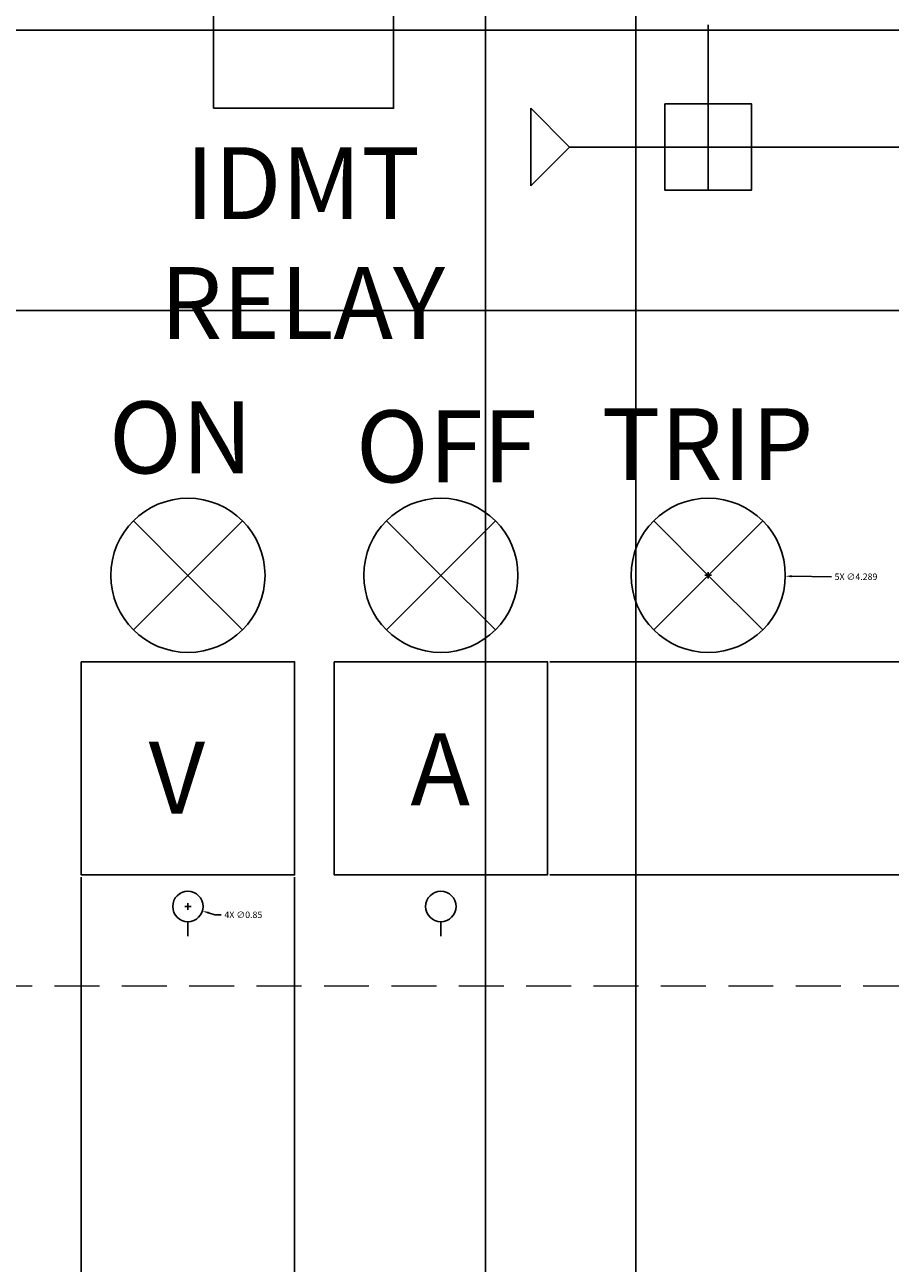
# Model space of a CAD drawing. Units: inches. Extents: x 412 to 584, y 208 to 437.
# Tile 19 of 28: x 471 to 495, y 352 to 387. Entities that reach past the tile are written whole.
import ezdxf

# ---------------------------------------------------------------- set-up
doc = ezdxf.new("R2010")
doc.units = ezdxf.units.IN
doc.header["$MEASUREMENT"] = 0
doc.linetypes.add('HIDDEN', pattern=[0.375, 0.25, -0.125])
for name, color, linetype, lineweight in [('A-ANNO-DIMS', 2, 'Continuous', 18), ('E-ANNO-TEXT', 7, 'Continuous', 18), ('E-ENCL-HIDN', 3, 'HIDDEN', 18), ('E-POWR-EQPM', 3, 'Continuous', 25)]:
    doc.layers.add(name, color=color, linetype=linetype, lineweight=lineweight)
doc.styles.get("Standard").update_dxf_attribs({"font": 'arial.ttf'})
doc.dimstyles.get("Standard").update_dxf_attribs({"dimtxt": 0.18, "dimasz": 0.18, "dimexe": 0.18, "dimexo": 0.0625, "dimgap": 0.09, "dimtad": 0, "dimtih": 1, "dimtoh": 1, "dimdec": 4, "dimzin": 0, "dimdsep": 46, "dimtxsty": 'Standard', "dimcen": 0.09, "dimadec": 0, "dimazin": 0, "dimtfac": 1, "dimtdec": 4, "dimtofl": 0, "dimtmove": 0, "dimatfit": 3, "dimfxl": 1, "dimtolj": 1, "dimtzin": 0, "dimarcsym": 0})

# ---------------------------------------------------------------- blocks, each defined once
blk = doc.blocks.new('*U1')
blk.add_line((0.758, -0.758), (-0.758, 0.758))
blk = doc.blocks.new('*U2')
at = {"color": 0, "linetype": 'ByBlock', "lineweight": -2, "transparency": 16777216}
blk.add_blockref('*U1', (78.828, 13.791), dxfattribs=at)
for p, rotation in [((80.344, 13.791), 269.9999999999999), ((78.828, 12.275), 89.99999999999996), ((80.344, 12.275), 180)]:
    blk.add_blockref('*U1', p, dxfattribs=dict(at, rotation=rotation))
blk = doc.blocks.new('INDICATOR-LAMP')
blk.add_circle((2.145, 2.145), 2.145)
at = {"rotation": 90.00000000000003}
blk.add_blockref('*U2', (15.178, -77.441), dxfattribs=at)
blk = doc.blocks.new('METER-VA')
blk.add_line((2.966, 0.398), (2.966, 0))
blk.add_lwpolyline([(0, 7.63), (5.932, 7.63), (5.932, 1.698), (0, 1.698)], close=True)
blk.add_circle((2.966, 0.821), 0.423)
blk = doc.blocks.new('*D23')
at = {"layer": 'A-ANNO-DIMS', "color": 0, "lineweight": -2, "transparency": 16777216}
for p, q in [((466.041, 360.196), (412.276, 360.196)), ((412.456, 360.016), (412.456, 354.967)), ((412.456, 349.553), (412.456, 354.603)), ((499.225, 349.373), (412.276, 349.373))]:
    blk.add_line(p, q, dxfattribs=at)
at = {"layer": 'A-ANNO-DIMS', "color": 0, "transparency": 16777216}
for points in [[(412.426, 360.016), (412.486, 360.016), (412.456, 360.196)], [(412.426, 349.553), (412.486, 349.553), (412.456, 349.373)]]:
    blk.add_solid(points, dxfattribs=at)
at = {"layer": 'Defpoints', "color": 0, "transparency": 16777216}
for p in [(466.104, 360.196), (412.456, 349.373), (499.288, 349.373)]:
    blk.add_point(p, dxfattribs=at)
at = {"layer": 'A-ANNO-DIMS', "color": 0, "transparency": 16777216, "insert": (412.456, 354.785), "char_height": 0.18, "attachment_point": 5}
blk.add_mtext('\\A1;10.823', dxfattribs=at)
blk = doc.blocks.new('*D28')
at = {"layer": 'A-ANNO-DIMS', "color": 0, "lineweight": -2, "transparency": 16777216}
for p, q in [((450.562, 256.635), (450.562, 437.465)), ((450.742, 437.285), (502.724, 437.285)), ((555.616, 437.285), (503.634, 437.285)), ((555.796, 256.635), (555.796, 437.465))]:
    blk.add_line(p, q, dxfattribs=at)
at = {"layer": 'A-ANNO-DIMS', "color": 0, "transparency": 16777216}
for points in [[(450.742, 437.315), (450.742, 437.255), (450.562, 437.285)], [(555.616, 437.315), (555.616, 437.255), (555.796, 437.285)]]:
    blk.add_solid(points, dxfattribs=at)
at = {"layer": 'Defpoints', "color": 0, "transparency": 16777216}
for p in [(555.796, 437.285), (450.562, 256.573), (555.796, 256.573)]:
    blk.add_point(p, dxfattribs=at)
at = {"layer": 'A-ANNO-DIMS', "color": 0, "transparency": 16777216, "insert": (503.179, 437.285), "char_height": 0.18, "attachment_point": 5}
blk.add_mtext('\\A1;105.23', dxfattribs=at)
blk = doc.blocks.new('*D30')
at = {"layer": 'A-ANNO-DIMS', "color": 0, "lineweight": -2, "transparency": 16777216}
for p, q in [((495.864, 386.793), (412.276, 386.793)), ((412.456, 386.613), (412.456, 383.072)), ((412.456, 379.167), (412.456, 382.708)), ((495.864, 378.987), (412.276, 378.987))]:
    blk.add_line(p, q, dxfattribs=at)
at = {"layer": 'A-ANNO-DIMS', "color": 0, "transparency": 16777216}
for points in [[(412.426, 386.613), (412.486, 386.613), (412.456, 386.793)], [(412.426, 379.167), (412.486, 379.167), (412.456, 378.987)]]:
    blk.add_solid(points, dxfattribs=at)
at = {"layer": 'Defpoints', "color": 0, "transparency": 16777216}
for p in [(495.927, 386.793), (412.456, 378.987), (495.927, 378.987)]:
    blk.add_point(p, dxfattribs=at)
at = {"layer": 'A-ANNO-DIMS', "color": 0, "transparency": 16777216, "insert": (412.456, 382.89), "char_height": 0.18, "attachment_point": 5}
blk.add_mtext('\\A1;7.807', dxfattribs=at)
blk = doc.blocks.new('*D33')
at = {"layer": 'A-ANNO-DIMS', "color": 0, "lineweight": -2, "transparency": 16777216}
for p, q in [((472.49, 363.226), (472.49, 208.233)), ((478.422, 363.226), (478.422, 208.233)), ((472.67, 208.413), (475.064, 208.413)), ((478.242, 208.413), (475.849, 208.413))]:
    blk.add_line(p, q, dxfattribs=at)
at = {"layer": 'A-ANNO-DIMS', "color": 0, "transparency": 16777216}
for points in [[(472.67, 208.443), (472.67, 208.383), (472.49, 208.413)], [(478.242, 208.443), (478.242, 208.383), (478.422, 208.413)]]:
    blk.add_solid(points, dxfattribs=at)
at = {"layer": 'Defpoints', "color": 0, "transparency": 16777216}
for p in [(472.49, 363.289), (478.422, 363.289), (478.422, 208.413)]:
    blk.add_point(p, dxfattribs=at)
at = {"layer": 'A-ANNO-DIMS', "color": 0, "transparency": 16777216, "insert": (475.456, 208.413), "char_height": 0.18, "attachment_point": 5}
blk.add_mtext('\\A1;5.932', dxfattribs=at)
blk = doc.blocks.new('*D35')
at = {"layer": 'A-ANNO-DIMS', "color": 0, "lineweight": -2, "transparency": 16777216}
for p, q in [((485.523, 369.221), (583.674, 369.221)), ((583.494, 369.041), (583.494, 366.437)), ((583.494, 363.469), (583.494, 366.073)), ((485.523, 363.289), (583.674, 363.289))]:
    blk.add_line(p, q, dxfattribs=at)
at = {"layer": 'A-ANNO-DIMS', "color": 0, "transparency": 16777216}
for points in [[(583.464, 369.041), (583.524, 369.041), (583.494, 369.221)], [(583.464, 363.469), (583.524, 363.469), (583.494, 363.289)]]:
    blk.add_solid(points, dxfattribs=at)
at = {"layer": 'Defpoints', "color": 0, "transparency": 16777216}
for p in [(485.46, 369.221), (485.46, 363.289), (583.494, 363.289)]:
    blk.add_point(p, dxfattribs=at)
at = {"layer": 'A-ANNO-DIMS', "color": 0, "transparency": 16777216, "insert": (583.494, 366.255), "char_height": 0.18, "attachment_point": 5}
blk.add_mtext('\\A1;5.932', dxfattribs=at)
blk = doc.blocks.new('*D41')
at = {"layer": 'A-ANNO-DIMS', "color": 0, "lineweight": -2, "transparency": 16777216}
for p, q in [((483.735, 316.045), (483.735, 437.465)), ((483.915, 437.285), (485.429, 437.285)), ((487.737, 437.285), (486.222, 437.285)), ((487.917, 316.045), (487.917, 437.465))]:
    blk.add_line(p, q, dxfattribs=at)
at = {"layer": 'A-ANNO-DIMS', "color": 0, "transparency": 16777216}
for points in [[(483.915, 437.315), (483.915, 437.255), (483.735, 437.285)], [(487.737, 437.315), (487.737, 437.255), (487.917, 437.285)]]:
    blk.add_solid(points, dxfattribs=at)
at = {"layer": 'Defpoints', "color": 0, "transparency": 16777216}
for p in [(487.917, 437.285), (483.735, 315.982), (487.917, 315.982)]:
    blk.add_point(p, dxfattribs=at)
at = {"layer": 'A-ANNO-DIMS', "color": 0, "transparency": 16777216, "insert": (485.826, 437.285), "char_height": 0.18, "attachment_point": 5}
blk.add_mtext('\\A1;4.182', dxfattribs=at)
blk = doc.blocks.new('*D43')
at = {"layer": 'A-ANNO-DIMS', "color": 0, "lineweight": -2, "transparency": 16777216}
for p, q in [((489.842, 371.624), (490.022, 371.624)), ((489.932, 371.534), (489.932, 371.714)), ((493.363, 371.585), (492.256, 371.598))]:
    blk.add_line(p, q, dxfattribs=at)
at = {"layer": 'A-ANNO-DIMS', "color": 0, "transparency": 16777216}
blk.add_solid([(492.257, 371.628), (492.256, 371.568), (492.076, 371.6)], dxfattribs=at)
at = {"layer": 'Defpoints', "color": 0, "transparency": 16777216}
for p in [(487.788, 371.648), (492.076, 371.6)]:
    blk.add_point(p, dxfattribs=at)
at = {"layer": 'A-ANNO-DIMS', "color": 0, "transparency": 16777216, "insert": (494.044, 371.585), "char_height": 0.18, "attachment_point": 5}
blk.add_mtext('\\A1;5X ∅4.289', dxfattribs=at)
blk = doc.blocks.new('*D49')
at = {"layer": 'A-ANNO-DIMS', "color": 0, "lineweight": -2, "transparency": 16777216}
for p, q in [((475.456, 362.322), (475.456, 362.502)), ((475.366, 362.412), (475.546, 362.412)), ((476.205, 362.181), (476.033, 362.234)), ((476.385, 362.181), (476.205, 362.181))]:
    blk.add_line(p, q, dxfattribs=at)
at = {"layer": 'A-ANNO-DIMS', "color": 0, "transparency": 16777216}
blk.add_solid([(476.041, 362.263), (476.024, 362.206), (475.861, 362.287)], dxfattribs=at)
at = {"layer": 'Defpoints', "color": 0, "transparency": 16777216}
for p in [(475.052, 362.538), (475.861, 362.287)]:
    blk.add_point(p, dxfattribs=at)
at = {"layer": 'A-ANNO-DIMS', "color": 0, "transparency": 16777216, "insert": (476.999, 362.181), "char_height": 0.18, "attachment_point": 5}
blk.add_mtext('\\A1;4X ∅0.85', dxfattribs=at)

msp = doc.modelspace()

# ---------------------------------------------------------------- linework, layer by layer
at = {"layer": 'E-ENCL-HIDN', "ltscale": 5}
msp.add_lwpolyline([(466.1037, 400.175), (538.6186, 400.175), (538.6186, 360.1961), (466.1037, 360.1961)], close=True, dxfattribs=at)
at = {"layer": 'E-POWR-EQPM'}
for p, q in [((489.932, 382.3348), (489.932, 386.939)), ((486.0745, 383.5382), (484.9955, 384.6173)), ((484.9955, 382.4592), (484.9955, 384.6173)), ((486.0745, 383.5382), (484.9955, 382.4592)), ((490.5891, 383.5382), (486.0745, 383.5382)), ((498.5775, 383.5382), (490.5891, 383.5382))]:
    msp.add_line(p, q, dxfattribs=at)
for points in [[(476.1684, 384.6173), (481.1791, 384.6173), (481.1791, 388.3577), (476.1684, 388.3577)], [(488.7286, 384.7417), (491.1355, 384.7417), (491.1355, 382.3348), (488.7286, 382.3348)]]:
    msp.add_lwpolyline(points, close=True, dxfattribs=at)

# ---------------------------------------------------------------- block references
at = {"layer": 'E-POWR-EQPM', "rotation": 270}
for p in [(473.3118, 373.7686), (480.3498, 373.7686), (487.7874, 373.7686)]:
    msp.add_blockref('INDICATOR-LAMP', p, dxfattribs=at)
at = {"layer": 'E-POWR-EQPM'}
for p in [(472.49, 361.591), (479.528, 361.591)]:
    msp.add_blockref('METER-VA', p, dxfattribs=at)

# ---------------------------------------------------------------- texts
at = {"layer": 'E-ANNO-TEXT', "char_height": 2, "attachment_point": 1}
for s, width, heights, insert in [('\\pxqc;IDMT\\PRELAY', 14.172159, [6.5789], (471.5606, 383.533)), ('\\pxqc;ON', 13.633448, [2.9648], (468.4413, 376.4612)), ('\\pxqc;OFF', 13.633448, [2.9648], (475.8321, 376.2109)), ('\\pxqc;TRIP', 13.633448, [2.9648], (483.0976, 376.2735)), ('\\pxqc;V', 13.633448, [2.9648], (468.3315, 366.9952)), ('\\pxqc;A', 13.633448, [2.9648], (475.659, 367.2276))]:
    msp.add_mtext_dynamic_manual_height_columns(s, width=width, gutter_width=1, heights=heights, dxfattribs=dict(at, insert=insert))

# ---------------------------------------------------------------- dimensions: what is measured, and where the dimension line sits
at = {"layer": 'A-ANNO-DIMS'}
for base, p1, p2, override, picture, middle in [((555.7959, 437.2847), (450.562, 256.5729), (555.7959, 256.5729), {"dimdec": 2, "dimlfac": 1, "dimrnd": 0, "dimzin": 0, "dimdsep": 46, "dimlunit": 2}, '*D28', (503.1789, 437.2847)), ((487.9167, 437.2847), (483.7347, 315.9821), (487.9167, 315.9821), {"dimdec": 3, "dimlfac": 1, "dimrnd": 0, "dimzin": 0, "dimdsep": 46, "dimlunit": 2}, '*D41', (485.8257, 437.2847)), ((478.4225, 208.4133), (472.4903, 363.2888), (478.4225, 363.2888), {"dimdec": 3, "dimlfac": 1, "dimrnd": 0, "dimzin": 0, "dimdsep": 46, "dimlunit": 2}, '*D33', (475.4564, 208.4133))]:
    dim = msp.add_linear_dim(base=base, p1=p1, p2=p2, dimstyle='Standard', override=override, dxfattribs=at)
    dim.commit()
    dim.dimension.update_dxf_attribs({"geometry": picture, "text_midpoint": middle})
for base, p1, p2, picture, middle in [((412.4562, 378.9867), (495.9268, 386.7933), (495.9268, 378.9867), '*D30', (412.4562, 382.89)), ((583.4937, 363.2888), (485.4605, 369.221), (485.4605, 363.2888), '*D35', (583.4937, 366.2549)), ((412.4562, 349.3734), (466.1037, 360.1961), (499.2878, 349.3734), '*D23', (412.4562, 354.7847))]:
    dim = msp.add_linear_dim(base=base, p1=p1, p2=p2, angle=90, dimstyle='Standard', override={"dimdec": 3, "dimlfac": 1, "dimrnd": 0, "dimzin": 0, "dimdsep": 46, "dimlunit": 2}, dxfattribs=at)
    dim.commit()
    dim.dimension.update_dxf_attribs({"geometry": picture, "text_midpoint": middle})
for p1, p2, text, override, picture, middle in [((487.7875, 371.6475), (492.0765, 371.5997), '5X <>', {"dimdec": 3, "dimlfac": 1, "dimrnd": 0, "dimzin": 0, "dimdsep": 46, "dimlunit": 2}, '*D43', (493.3632, 371.5854)), ((475.0521, 362.5375), (475.8607, 362.2874), '4X <>', {"dimdec": 2, "dimlfac": 1, "dimrnd": 0, "dimzin": 0, "dimdsep": 46, "dimlunit": 2}, '*D49', (476.9992, 362.181))]:
    dim = msp.add_diameter_dim_2p(p1=p1, p2=p2, text=text, dimstyle='Standard', override=override, dxfattribs=at)
    dim.commit()
    dim.dimension.update_dxf_attribs({"geometry": picture, "text_midpoint": middle, "dimtype": 163})

doc.saveas('drawing.dxf')
